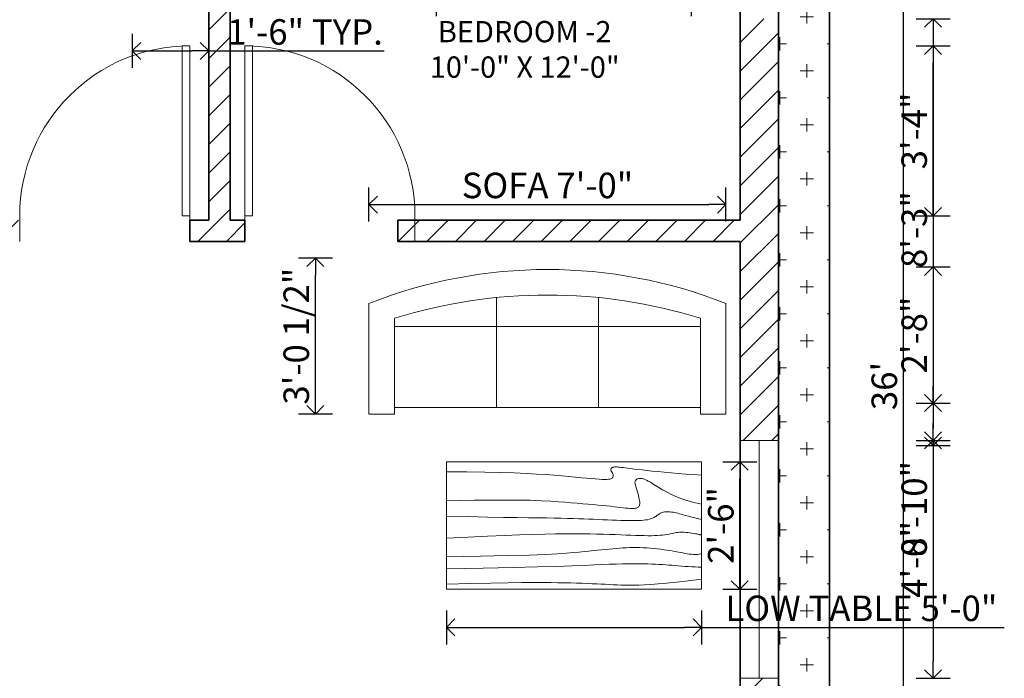
# Model space of a CAD drawing. Units: inches. Extents: x 686 to 1065, y 83 to 664.
# Tile 4 of 5: x 833 to 1065, y 308 to 463. Entities that reach past the tile are written whole.
import ezdxf

# ---------------------------------------------------------------- set-up
doc = ezdxf.new("R2010")
doc.units = ezdxf.units.IN
for name, color, linetype, lineweight in [('A-ANNO-DIMS', 2, 'Continuous', 18), ('A-AREA-IDEN', 7, 'Continuous', 20), ('A-DOOR', 4, 'Continuous', 20), ('A-FURN', 8, 'Continuous', 18), ('A-GLAZ', 172, 'Continuous', 18), ('A-WALL', 7, 'Continuous', 35), ('A-WALL-PATT', 253, 'Continuous', 13), ('C-PROP', 7, 'Continuous', 35), ('L-SITE-PATT', 94, 'Continuous', 13)]:
    doc.layers.add(name, color=color, linetype=linetype, lineweight=lineweight)
doc.styles.get("Standard").update_dxf_attribs({"font": 'arial.ttf'})
doc.dimstyles.new('ISO-25', dxfattribs={"dimtxt": 6, "dimasz": 4, "dimexe": 4, "dimexo": 4, "dimtad": 1, "dimdec": 1, "dimlunit": 3, "dimtxsty": 'Standard', "dimblk": 'OPEN90', "dimcen": 2.5, "dimadec": 0, "dimazin": 0, "dimtfac": 1, "dimtdec": 1, "dimtmove": 0, "dimatfit": 3, "dimfxl": 4, "dimfxlon": 1, "dimarcsym": 0})

# ---------------------------------------------------------------- blocks, each defined once
blk = doc.blocks.new('Sofa - Roundback 7 ft.')
for p, q in [((-12.00002, -32.4421), (-12.00003, -6.5971)), ((11.99997, -32.4421), (11.99998, -6.5971)), ((-36.000027, -34), (-36.000027, -11.4696)), ((35.99998, -34), (35.99998, -11.4696)), ((-35.999844, -13.3819), (35.9998, -13.3819)), ((-36.000027, -32.4421), (35.99998, -32.4421))]:
    blk.add_line(p, q)
for points in [[(-36.000027, -34), (-42.000027, -34), (-42.000027, -8)], [(41.99998, -8), (41.99998, -34), (35.99998, -34)]]:
    blk.add_lwpolyline(points)
for centre, radius, start, end in [((0, -114.25), 114.25, 68.43141, 111.5686), ((-0.00001, -127.1968), 121.1968, 72.72033, 107.2797)]:
    blk.add_arc(centre, radius, start, end)
blk = doc.blocks.new('Table - Rectangular Woodgrain 60 x 30 in.')
for p, q in [((0, 0), (0, -30)), ((60, 0), (0, 0)), ((60, -30), (60, 0)), ((0, -30), (60, -30))]:
    blk.add_line(p, q)
for points in [[(0, -2.4), (4.8155, -2.418), (9.0302, -2.4688), (12.709, -2.5477), (15.9167, -2.65), (18.7181, -2.7711), (21.1781, -2.9063), (23.3616, -3.0508), (25.3333, -3.2), (27.1477, -3.3495), (28.8172, -3.4958), (30.3437, -3.636), (31.7291, -3.7667), (32.9756, -3.8849), (34.0849, -3.9875), (35.059, -4.0714), (35.9, -4.1334), (36.6114, -4.1711), (37.2041, -4.1854), (37.6906, -4.1779), (38.0833, -4.15), (38.3948, -4.1034), (38.6375, -4.0396), (38.8239, -3.9602), (38.9666, -3.8667), (39.0764, -3.7608), (39.1573, -3.6448), (39.2116, -3.521), (39.2416, -3.3917), (39.2498, -3.2593), (39.2385, -3.1261), (39.21, -2.9944), (39.1666, -2.8667), (39.111, -2.7447), (39.0468, -2.6281), (38.978, -2.5163), (38.9083, -2.4083), (38.8418, -2.3035), (38.7823, -2.201), (38.7337, -2.1001), (38.7, -2), (38.6844, -1.9003), (38.6875, -1.8021), (38.7094, -1.707), (38.75, -1.6167), (38.8094, -1.5326), (38.8875, -1.4563), (38.9844, -1.3893), (39.1, -1.3333), (39.2351, -1.2896), (39.3937, -1.2583), (39.5804, -1.2396), (39.8, -1.2333), (40.057, -1.2396), (40.3562, -1.2583), (40.7023, -1.2896), (41.1, -1.3333), (41.5547, -1.3895), (42.0755, -1.4573), (42.6721, -1.5361), (43.3542, -1.625), (44.1316, -1.7233), (45.014, -1.8302), (46.0114, -1.9449), (47.1333, -2.0667), (48.3862, -2.1947), (49.7625, -2.3281), (51.2513, -2.4663), (52.8416, -2.6083), (54.5226, -2.7535), (56.2833, -2.9011), (58.1127, -3.0501), (60, -3.2)], [(0, -9.2), (6.5759, -9.0858), (11.9385, -9.0365), (16.2527, -9.0418), (19.6833, -9.0917), (22.3952, -9.1759), (24.5531, -9.2844), (26.322, -9.4069), (27.8666, -9.5333), (29.3241, -9.6553), (30.7203, -9.7719), (32.0532, -9.8837), (33.3208, -9.9917), (34.5213, -10.0965), (35.6526, -10.199), (36.7128, -10.2999), (37.7, -10.4), (38.6129, -10.4996), (39.4531, -10.5969), (40.223, -10.6895), (40.925, -10.775), (41.5613, -10.8512), (42.1344, -10.9156), (42.6465, -10.966), (43.1, -11), (43.4976, -11.0158), (43.8437, -11.0136), (44.143, -10.9942), (44.4, -10.9583), (44.6195, -10.9069), (44.8062, -10.8406), (44.9648, -10.7603), (45.1, -10.6667), (45.2155, -10.5598), (45.3114, -10.4365), (45.3871, -10.2929), (45.4416, -10.125), (45.4743, -9.929), (45.4844, -9.7011), (45.4709, -9.4371), (45.4333, -9.1333), (45.3716, -8.7883), (45.2896, -8.4104), (45.1919, -8.0107), (45.0833, -7.6), (44.9685, -7.1893), (44.8521, -6.7896), (44.7388, -6.4117), (44.6333, -6.0667), (44.54, -5.7628), (44.4614, -5.4979), (44.4001, -5.2675), (44.3583, -5.0667), (44.3384, -4.8909), (44.3427, -4.7354), (44.3736, -4.5956), (44.4333, -4.4667), (44.5236, -4.3453), (44.6427, -4.2333), (44.7884, -4.1339), (44.9583, -4.05), (45.1501, -3.9849), (45.3614, -3.9417), (45.59, -3.9234), (45.8333, -3.9333), (46.0915, -3.9749), (46.3734, -4.0531), (46.6906, -4.1736), (47.0542, -4.3417), (47.4756, -4.5629), (47.9661, -4.8427), (48.5372, -5.1866), (49.2, -5.6), (49.9676, -6.0844), (50.8594, -6.625), (51.8965, -7.2031), (53.1, -7.8), (54.491, -8.3969), (56.0906, -8.975), (57.9199, -9.5156), (60, -10)], [(0, -12.8), (5.1847, -12.9322), (9.6213, -13.0323), (13.3963, -13.1059), (16.5958, -13.1583), (19.3063, -13.1952), (21.614, -13.2219), (23.6054, -13.2439), (25.3666, -13.2667), (26.9728, -13.2947), (28.4531, -13.3281), (29.8256, -13.3663), (31.1083, -13.4083), (32.3191, -13.4535), (33.476, -13.501), (34.597, -13.5501), (35.7, -13.6), (36.7984, -13.6497), (37.8875, -13.6979), (38.9578, -13.743), (40, -13.7833), (41.0047, -13.8174), (41.9625, -13.8438), (42.864, -13.8607), (43.7, -13.8667), (44.4631, -13.8604), (45.1552, -13.8417), (45.7801, -13.8104), (46.3416, -13.7667), (46.8439, -13.7104), (47.2906, -13.6417), (47.6858, -13.5604), (48.0333, -13.4667), (48.3375, -13.3608), (48.6042, -13.2448), (48.8396, -13.121), (49.05, -12.9917), (49.2417, -12.8593), (49.4208, -12.7261), (49.5937, -12.5944), (49.7667, -12.4667), (49.9452, -12.3451), (50.1323, -12.2313), (50.3303, -12.1268), (50.5416, -12.0333), (50.7686, -11.9524), (51.0135, -11.8854), (51.2788, -11.8341), (51.5666, -11.8), (51.8785, -11.7843), (52.2116, -11.7865), (52.562, -11.8059), (52.926, -11.8417), (53.2998, -11.8931), (53.6795, -11.9594), (54.0614, -12.0397), (54.4416, -12.1333), (54.8223, -12.2401), (55.2293, -12.3625), (55.6942, -12.5037), (56.2489, -12.6667), (56.9251, -12.8547), (57.7545, -13.0708), (58.7689, -13.3182), (60, -13.6)], [(0, -18), (5.124, -17.7273), (9.6609, -17.5057), (13.6705, -17.3303), (17.2125, -17.1958), (20.3467, -17.0973), (23.1328, -17.0297), (25.6307, -16.9878), (27.9, -16.9667), (29.9928, -16.9617), (31.9302, -16.9703), (33.7254, -16.9907), (35.3917, -17.0208), (36.9423, -17.0588), (38.3906, -17.1026), (39.7499, -17.1503), (41.0333, -17.2), (42.2519, -17.2496), (43.4073, -17.2969), (44.4986, -17.3395), (45.525, -17.375), (46.4858, -17.4012), (47.3802, -17.4156), (48.2074, -17.416), (48.9667, -17.4), (49.6583, -17.3662), (50.2872, -17.3167), (50.8595, -17.2547), (51.3812, -17.1833), (51.8584, -17.1057), (52.2971, -17.025), (52.7034, -16.9443), (53.0833, -16.8667), (53.443, -16.7951), (53.789, -16.7313), (54.128, -16.6768), (54.4666, -16.6334), (54.8115, -16.6024), (55.1693, -16.5854), (55.5465, -16.5841), (55.95, -16.6), (56.3828, -16.6337), (56.8346, -16.6823), (57.2915, -16.7418), (57.7396, -16.8084), (58.165, -16.878), (58.5539, -16.9469), (58.8924, -17.0111), (59.1666, -17.0667), (59.3679, -17.1107), (59.5078, -17.1438), (59.6032, -17.1675), (59.6708, -17.1833), (59.7275, -17.193), (59.7901, -17.1979), (59.8753, -17.1998), (60, -17.2)], [(0, -22.4), (8.0098, -22.2501), (14.4094, -22.1011), (19.4168, -21.9535), (23.25, -21.8083), (26.1269, -21.6663), (28.2656, -21.5281), (29.884, -21.3947), (31.2, -21.2667), (32.3967, -21.1448), (33.5172, -21.0292), (34.5697, -20.9198), (35.5625, -20.8167), (36.5037, -20.7198), (37.4015, -20.6292), (38.2642, -20.5448), (39.1, -20.4667), (39.9164, -20.3951), (40.7187, -20.3313), (41.5117, -20.2768), (42.3, -20.2333), (43.0883, -20.2024), (43.8812, -20.1854), (44.6836, -20.1841), (45.5, -20.2), (46.3328, -20.234), (47.1747, -20.2844), (48.0163, -20.3488), (48.8479, -20.425), (49.66, -20.5106), (50.4429, -20.6031), (51.1872, -20.7004), (51.8833, -20.8), (52.5246, -20.8999), (53.1166, -20.9995), (53.6681, -21.0983), (54.1875, -21.1958), (54.6834, -21.2919), (55.1646, -21.3859), (55.6394, -21.4777), (56.1167, -21.5667), (56.6028, -21.6515), (57.0961, -21.7266), (57.5929, -21.7852), (58.0896, -21.8208), (58.5823, -21.8268), (59.0674, -21.7964), (59.5412, -21.723), (60, -21.6)], [(0, -25.2), (8.6355, -25.0504), (15.7026, -24.9031), (21.4049, -24.7606), (25.9458, -24.625), (29.529, -24.4988), (32.3578, -24.3844), (34.6359, -24.284), (36.5667, -24.2), (38.3213, -24.1341), (39.9417, -24.0854), (41.437, -24.0523), (42.8167, -24.0333), (44.0901, -24.0268), (45.2667, -24.0313), (46.3557, -24.0451), (47.3667, -24.0667), (48.309, -24.0947), (49.1928, -24.1287), (50.0284, -24.168), (50.826, -24.2125), (51.5959, -24.2617), (52.3483, -24.3151), (53.0935, -24.3725), (53.8417, -24.4334), (54.6009, -24.497), (55.3699, -24.561), (56.1454, -24.6226), (56.9239, -24.6792), (57.7021, -24.7279), (58.4764, -24.7662), (59.2435, -24.7911), (60, -24.8)], [(0, -28.8), (5.6867, -28.6681), (10.45, -28.5698), (14.407, -28.5012), (17.675, -28.4584), (20.3711, -28.4374), (22.6125, -28.4344), (24.5164, -28.4455), (26.2, -28.4667), (27.762, -28.4947), (29.2276, -28.5281), (30.6033, -28.5663), (31.8958, -28.6084), (33.1118, -28.6535), (34.2578, -28.7011), (35.3405, -28.7501), (36.3666, -28.8), (37.3443, -28.8497), (38.288, -28.8974), (39.2137, -28.9412), (40.1375, -28.9792), (41.0753, -29.0093), (42.0432, -29.0297), (43.0572, -29.0384), (44.1333, -29.0333), (45.2936, -29.0114), (46.5843, -28.9641), (48.0579, -28.8816), (49.7666, -28.7542), (51.7629, -28.5721), (54.0989, -28.3255), (56.8272, -28.0048), (60, -27.6)]]:
    blk.add_lwpolyline(points)
blk = doc.blocks.new('_Open90')
at = {"color": 0, "linetype": 'ByBlock', "lineweight": -2}
for p, q in [((0, 0), (-1, 0)), ((-0.5, 0.5), (0, 0)), ((0, 0), (-0.5, -0.5))]:
    blk.add_line(p, q, dxfattribs=at)
blk = doc.blocks.new('*D8')
at = {"layer": 'A-ANNO-DIMS', "color": 0, "lineweight": -2, "transparency": 16777216}
for p, q in [((1036.76, 592.73), (1044.76, 592.73)), ((1040.76, 588.73), (1040.76, 164.73)), ((1036.76, 160.73), (1044.76, 160.73))]:
    blk.add_line(p, q, dxfattribs=at)
at = {"layer": 'Defpoints', "color": 0, "transparency": 16777216}
for p in [(1023.37, 592.73), (1023.37, 160.73), (1040.76, 160.73)]:
    blk.add_point(p, dxfattribs=at)
at = {"layer": 'A-ANNO-DIMS', "color": 0, "lineweight": -2, "transparency": 16777216, "xscale": 4, "yscale": 4, "zscale": 4}
for p, rotation in [((1040.76, 592.73), 90), ((1040.76, 160.73), 270)]:
    blk.add_blockref('_Open90', p, dxfattribs=dict(at, rotation=rotation))
at = {"layer": 'A-ANNO-DIMS', "color": 0, "transparency": 16777216, "insert": (1037.07, 376.73), "char_height": 6, "attachment_point": 5, "rotation": 90}
blk.add_mtext("36'", dxfattribs=at)
blk = doc.blocks.new('*U23')
for p, q in [((0, 0), (0, -6)), ((-40, 0), (-40, -6))]:
    blk.add_line(p, q)
blk.add_lwpolyline([(0, 0), (0, 40), (-1.75, 40), (-1.75, 0)], close=True)
blk.add_arc((0, 0), 40, 90, 180)
blk = doc.blocks.new('*D27')
at = {"layer": 'A-ANNO-DIMS', "color": 0, "lineweight": -2, "transparency": 16777216}
for p, q in [((930.83, 471.73), (930.83, 463.73)), ((990.83, 471.73), (990.83, 463.73)), ((986.83, 467.73), (934.83, 467.73))]:
    blk.add_line(p, q, dxfattribs=at)
at = {"layer": 'Defpoints', "color": 0, "transparency": 16777216}
for p in [(930.83, 479.73), (990.83, 479.73), (930.83, 467.73)]:
    blk.add_point(p, dxfattribs=at)
at = {"layer": 'A-ANNO-DIMS', "color": 0, "lineweight": -2, "transparency": 16777216, "xscale": 4, "yscale": 4, "zscale": 4, "rotation": 180}
blk.add_blockref('_Open90', (930.83, 467.73), dxfattribs=at)
at = {"layer": 'A-ANNO-DIMS', "color": 0, "lineweight": -2, "transparency": 16777216, "xscale": 4, "yscale": 4, "zscale": 4}
blk.add_blockref('_Open90', (990.83, 467.73), dxfattribs=at)
at = {"layer": 'A-ANNO-DIMS', "color": 0, "transparency": 16777216, "insert": (960.83, 471.42), "char_height": 6, "attachment_point": 5}
blk.add_mtext('5\'-0" TYP.', dxfattribs=at)
blk = doc.blocks.new('*D29')
at = {"layer": 'A-ANNO-DIMS', "color": 0, "lineweight": -2, "transparency": 16777216}
for p, q in [((859.37, 459.54), (859.37, 451.54)), ((877.37, 459.54), (877.37, 451.54)), ((863.37, 455.54), (873.37, 455.54)), ((877.37, 455.54), (918.63, 455.54))]:
    blk.add_line(p, q, dxfattribs=at)
at = {"layer": 'Defpoints', "color": 0, "transparency": 16777216}
for p in [(859.37, 468.63), (877.37, 468.63), (877.37, 455.54)]:
    blk.add_point(p, dxfattribs=at)
at = {"layer": 'A-ANNO-DIMS', "color": 0, "lineweight": -2, "transparency": 16777216, "xscale": 4, "yscale": 4, "zscale": 4, "rotation": 180}
blk.add_blockref('_Open90', (859.37, 455.54), dxfattribs=at)
at = {"layer": 'A-ANNO-DIMS', "color": 0, "lineweight": -2, "transparency": 16777216, "xscale": 4, "yscale": 4, "zscale": 4}
blk.add_blockref('_Open90', (877.37, 455.54), dxfattribs=at)
at = {"layer": 'A-ANNO-DIMS', "color": 0, "transparency": 16777216, "insert": (900, 459.23), "char_height": 6, "attachment_point": 5}
blk.add_mtext('1\'-6" TYP.', dxfattribs=at)
blk = doc.blocks.new('*D36')
at = {"layer": 'A-ANNO-DIMS', "color": 0, "lineweight": -2, "transparency": 16777216}
for p, q in [((915.04, 415.4), (915.04, 423.4)), ((999.04, 415.4), (999.04, 423.4)), ((919.04, 419.4), (995.04, 419.4))]:
    blk.add_line(p, q, dxfattribs=at)
at = {"layer": 'Defpoints', "color": 0, "transparency": 16777216}
for p in [(999.04, 419.4), (915.04, 406.8), (999.04, 406.8)]:
    blk.add_point(p, dxfattribs=at)
at = {"layer": 'A-ANNO-DIMS', "color": 0, "lineweight": -2, "transparency": 16777216, "xscale": 4, "yscale": 4, "zscale": 4, "rotation": 180}
blk.add_blockref('_Open90', (915.04, 419.4), dxfattribs=at)
at = {"layer": 'A-ANNO-DIMS', "color": 0, "lineweight": -2, "transparency": 16777216, "xscale": 4, "yscale": 4, "zscale": 4}
blk.add_blockref('_Open90', (999.04, 419.4), dxfattribs=at)
at = {"layer": 'A-ANNO-DIMS', "color": 0, "transparency": 16777216, "insert": (957.04, 423.13), "char_height": 6, "attachment_point": 5}
blk.add_mtext('SOFA 7\'-0"', dxfattribs=at)
blk = doc.blocks.new('*D37')
at = {"layer": 'A-ANNO-DIMS', "color": 0, "lineweight": -2, "transparency": 16777216}
for p, q in [((906.44, 406.8), (898.44, 406.8)), ((902.44, 374.13), (902.44, 402.8)), ((906.44, 370.13), (898.44, 370.13))]:
    blk.add_line(p, q, dxfattribs=at)
at = {"layer": 'Defpoints', "color": 0, "transparency": 16777216}
for p in [(902.44, 406.8), (915.04, 406.8), (915.04, 370.13)]:
    blk.add_point(p, dxfattribs=at)
at = {"layer": 'A-ANNO-DIMS', "color": 0, "lineweight": -2, "transparency": 16777216, "xscale": 4, "yscale": 4, "zscale": 4}
for p, rotation in [((902.44, 406.8), 90), ((902.44, 370.13), 270)]:
    blk.add_blockref('_Open90', p, dxfattribs=dict(at, rotation=rotation))
at = {"layer": 'A-ANNO-DIMS', "color": 0, "transparency": 16777216, "insert": (898.71, 388.46), "char_height": 6, "attachment_point": 5, "rotation": 90}
blk.add_mtext('3\'-0 1/2"', dxfattribs=at)
blk = doc.blocks.new('*D38')
at = {"layer": 'A-ANNO-DIMS', "color": 0, "lineweight": -2, "transparency": 16777216}
for p, q in [((933.28, 323.93), (933.28, 315.93)), ((993.28, 323.93), (993.28, 315.93)), ((937.28, 319.93), (989.28, 319.93)), ((993.28, 319.93), (1064.52, 319.93))]:
    blk.add_line(p, q, dxfattribs=at)
at = {"layer": 'Defpoints', "color": 0, "transparency": 16777216}
for p in [(933.28, 328.93), (993.28, 328.93), (993.28, 319.93)]:
    blk.add_point(p, dxfattribs=at)
at = {"layer": 'A-ANNO-DIMS', "color": 0, "lineweight": -2, "transparency": 16777216, "xscale": 4, "yscale": 4, "zscale": 4, "rotation": 180}
blk.add_blockref('_Open90', (933.28, 319.93), dxfattribs=at)
at = {"layer": 'A-ANNO-DIMS', "color": 0, "lineweight": -2, "transparency": 16777216, "xscale": 4, "yscale": 4, "zscale": 4}
blk.add_blockref('_Open90', (993.28, 319.93), dxfattribs=at)
at = {"layer": 'A-ANNO-DIMS', "color": 0, "transparency": 16777216, "insert": (1030.9, 323.66), "char_height": 6, "attachment_point": 5}
blk.add_mtext('LOW TABLE 5\'-0"', dxfattribs=at)
blk = doc.blocks.new('*D39')
at = {"layer": 'A-ANNO-DIMS', "color": 0, "lineweight": -2, "transparency": 16777216}
for p, q in [((998.28, 358.93), (1006.28, 358.93)), ((1002.28, 332.93), (1002.28, 354.93)), ((998.28, 328.93), (1006.28, 328.93))]:
    blk.add_line(p, q, dxfattribs=at)
at = {"layer": 'Defpoints', "color": 0, "transparency": 16777216}
for p in [(993.28, 358.93), (1002.28, 358.93), (993.28, 328.93)]:
    blk.add_point(p, dxfattribs=at)
at = {"layer": 'A-ANNO-DIMS', "color": 0, "lineweight": -2, "transparency": 16777216, "xscale": 4, "yscale": 4, "zscale": 4}
for p, rotation in [((1002.28, 358.93), 90), ((1002.28, 328.93), 270)]:
    blk.add_blockref('_Open90', p, dxfattribs=dict(at, rotation=rotation))
at = {"layer": 'A-ANNO-DIMS', "color": 0, "transparency": 16777216, "insert": (998.59, 343.93), "char_height": 6, "attachment_point": 5, "rotation": 90}
blk.add_mtext('2\'-6"', dxfattribs=at)
blk = doc.blocks.new('*D48')
at = {"layer": 'A-ANNO-DIMS', "color": 0, "lineweight": -2, "transparency": 16777216}
for p, q in [((1043.78, 463.11), (1051.78, 463.11)), ((1047.78, 459.11), (1047.78, 367.95)), ((1043.78, 363.95), (1051.78, 363.95))]:
    blk.add_line(p, q, dxfattribs=at)
at = {"layer": 'Defpoints', "color": 0, "transparency": 16777216}
for p in [(1011.37, 463.11), (1011.37, 363.95), (1047.78, 363.95)]:
    blk.add_point(p, dxfattribs=at)
at = {"layer": 'A-ANNO-DIMS', "color": 0, "lineweight": -2, "transparency": 16777216, "xscale": 4, "yscale": 4, "zscale": 4}
for p, rotation in [((1047.78, 463.11), 90), ((1047.78, 363.95), 270)]:
    blk.add_blockref('_Open90', p, dxfattribs=dict(at, rotation=rotation))
at = {"layer": 'A-ANNO-DIMS', "color": 0, "transparency": 16777216, "insert": (1044.09, 413.53), "char_height": 6, "attachment_point": 5, "rotation": 90}
blk.add_mtext('8\'-3"', dxfattribs=at)
blk = doc.blocks.new('*D49')
at = {"layer": 'A-ANNO-DIMS', "color": 0, "lineweight": -2, "transparency": 16777216}
for p, q in [((1043.78, 363.95), (1051.78, 363.95)), ((1047.78, 359.95), (1047.78, 311.98)), ((1043.78, 307.98), (1051.78, 307.98))]:
    blk.add_line(p, q, dxfattribs=at)
at = {"layer": 'Defpoints', "color": 0, "transparency": 16777216}
for p in [(1011.37, 363.95), (1011.37, 307.98), (1047.78, 307.98)]:
    blk.add_point(p, dxfattribs=at)
at = {"layer": 'A-ANNO-DIMS', "color": 0, "lineweight": -2, "transparency": 16777216, "xscale": 4, "yscale": 4, "zscale": 4}
for p, rotation in [((1047.78, 363.95), 90), ((1047.78, 307.98), 270)]:
    blk.add_blockref('_Open90', p, dxfattribs=dict(at, rotation=rotation))
at = {"layer": 'A-ANNO-DIMS', "color": 0, "transparency": 16777216, "insert": (1044.09, 335.96), "char_height": 6, "attachment_point": 5, "rotation": 90}
blk.add_mtext('4\'-8"', dxfattribs=at)
blk = doc.blocks.new('*D54')
at = {"layer": 'A-ANNO-DIMS', "color": 0, "lineweight": -2, "transparency": 16777216}
for p, q in [((832.87, 613.14), (832.87, 621.14)), ((872.87, 613.14), (872.87, 621.14)), ((836.87, 617.14), (868.87, 617.14))]:
    blk.add_line(p, q, dxfattribs=at)
at = {"layer": 'Defpoints', "color": 0, "transparency": 16777216}
for p in [(872.87, 617.14), (832.87, 415.73), (872.87, 415.73)]:
    blk.add_point(p, dxfattribs=at)
at = {"layer": 'A-ANNO-DIMS', "color": 0, "lineweight": -2, "transparency": 16777216, "xscale": 4, "yscale": 4, "zscale": 4, "rotation": 180}
blk.add_blockref('_Open90', (832.87, 617.14), dxfattribs=at)
at = {"layer": 'A-ANNO-DIMS', "color": 0, "lineweight": -2, "transparency": 16777216, "xscale": 4, "yscale": 4, "zscale": 4}
blk.add_blockref('_Open90', (872.87, 617.14), dxfattribs=at)
at = {"layer": 'A-ANNO-DIMS', "color": 0, "transparency": 16777216, "insert": (852.87, 620.83), "char_height": 6, "attachment_point": 5}
blk.add_mtext('3\'-4"', dxfattribs=at)
blk = doc.blocks.new('*D55')
at = {"layer": 'A-ANNO-DIMS', "color": 0, "lineweight": -2, "transparency": 16777216}
for p, q in [((885.87, 613.14), (885.87, 621.14)), ((921.87, 613.14), (921.87, 621.14)), ((889.87, 617.14), (917.87, 617.14))]:
    blk.add_line(p, q, dxfattribs=at)
at = {"layer": 'Defpoints', "color": 0, "transparency": 16777216}
for p in [(921.87, 617.14), (885.87, 415.73), (921.87, 415.73)]:
    blk.add_point(p, dxfattribs=at)
at = {"layer": 'A-ANNO-DIMS', "color": 0, "lineweight": -2, "transparency": 16777216, "xscale": 4, "yscale": 4, "zscale": 4, "rotation": 180}
blk.add_blockref('_Open90', (885.87, 617.14), dxfattribs=at)
at = {"layer": 'A-ANNO-DIMS', "color": 0, "lineweight": -2, "transparency": 16777216, "xscale": 4, "yscale": 4, "zscale": 4}
blk.add_blockref('_Open90', (921.87, 617.14), dxfattribs=at)
at = {"layer": 'A-ANNO-DIMS', "color": 0, "transparency": 16777216, "insert": (903.87, 620.83), "char_height": 6, "attachment_point": 5}
blk.add_mtext('3\'-0"', dxfattribs=at)
blk = doc.blocks.new('*D56')
at = {"layer": 'A-ANNO-DIMS', "color": 0, "lineweight": -2, "transparency": 16777216}
for p, q in [((900.37, 613.14), (900.37, 621.14)), ((930.37, 613.14), (930.37, 621.14)), ((904.37, 617.14), (926.37, 617.14))]:
    blk.add_line(p, q, dxfattribs=at)
at = {"layer": 'Defpoints', "color": 0, "transparency": 16777216}
for p in [(930.37, 617.14), (900.37, 246.73), (930.37, 246.73)]:
    blk.add_point(p, dxfattribs=at)
at = {"layer": 'A-ANNO-DIMS', "color": 0, "lineweight": -2, "transparency": 16777216, "xscale": 4, "yscale": 4, "zscale": 4, "rotation": 180}
blk.add_blockref('_Open90', (900.37, 617.14), dxfattribs=at)
at = {"layer": 'A-ANNO-DIMS', "color": 0, "lineweight": -2, "transparency": 16777216, "xscale": 4, "yscale": 4, "zscale": 4}
blk.add_blockref('_Open90', (930.37, 617.14), dxfattribs=at)
at = {"layer": 'A-ANNO-DIMS', "color": 0, "transparency": 16777216, "insert": (915.37, 620.83), "char_height": 6, "attachment_point": 5}
blk.add_mtext('2\'-6"', dxfattribs=at)
blk = doc.blocks.new('*D57')
at = {"layer": 'A-ANNO-DIMS', "color": 0, "lineweight": -2, "transparency": 16777216}
for p, q in [((1043.78, 404.73), (1051.78, 404.73)), ((1047.78, 400.73), (1047.78, 376.73)), ((1043.78, 372.73), (1051.78, 372.73))]:
    blk.add_line(p, q, dxfattribs=at)
at = {"layer": 'Defpoints', "color": 0, "transparency": 16777216}
for p in [(828.37, 404.73), (828.37, 372.73), (1047.78, 372.73)]:
    blk.add_point(p, dxfattribs=at)
at = {"layer": 'A-ANNO-DIMS', "color": 0, "lineweight": -2, "transparency": 16777216, "xscale": 4, "yscale": 4, "zscale": 4}
for p, rotation in [((1047.78, 404.73), 90), ((1047.78, 372.73), 270)]:
    blk.add_blockref('_Open90', p, dxfattribs=dict(at, rotation=rotation))
at = {"layer": 'A-ANNO-DIMS', "color": 0, "transparency": 16777216, "insert": (1044.09, 388.73), "char_height": 6, "attachment_point": 5, "rotation": 90}
blk.add_mtext('2\'-8"', dxfattribs=at)
blk = doc.blocks.new('*D61')
at = {"layer": 'A-ANNO-DIMS', "color": 0, "lineweight": -2, "transparency": 16777216}
for p, q in [((1043.78, 372.73), (1051.78, 372.73)), ((1047.78, 368.73), (1047.78, 366.73)), ((1043.78, 362.73), (1051.78, 362.73)), ((1047.78, 362.73), (1047.78, 336.87))]:
    blk.add_line(p, q, dxfattribs=at)
at = {"layer": 'Defpoints', "color": 0, "transparency": 16777216}
for p in [(823.37, 372.73), (823.37, 362.73), (1047.78, 362.73)]:
    blk.add_point(p, dxfattribs=at)
at = {"layer": 'A-ANNO-DIMS', "color": 0, "lineweight": -2, "transparency": 16777216, "xscale": 4, "yscale": 4, "zscale": 4}
for p, rotation in [((1047.78, 372.73), 90), ((1047.78, 362.73), 270)]:
    blk.add_blockref('_Open90', p, dxfattribs=dict(at, rotation=rotation))
at = {"layer": 'A-ANNO-DIMS', "color": 0, "transparency": 16777216, "insert": (1044.09, 347.8), "char_height": 6, "attachment_point": 5, "rotation": 90}
blk.add_mtext('0\'-10"', dxfattribs=at)
blk = doc.blocks.new('*D63')
at = {"layer": 'A-ANNO-DIMS', "color": 0, "lineweight": -2, "transparency": 16777216}
for p, q in [((823.37, 92.32), (823.37, 84.32)), ((828.37, 92.32), (828.37, 84.32)), ((819.37, 88.32), (815.37, 88.32)), ((823.37, 88.32), (828.37, 88.32)), ((832.37, 88.32), (853.57, 88.32))]:
    blk.add_line(p, q, dxfattribs=at)
at = {"layer": 'Defpoints', "color": 0, "transparency": 16777216}
for p in [(823.37, 362.73), (828.37, 357.73), (828.37, 88.32)]:
    blk.add_point(p, dxfattribs=at)
at = {"layer": 'A-ANNO-DIMS', "color": 0, "lineweight": -2, "transparency": 16777216, "xscale": 4, "yscale": 4, "zscale": 4}
blk.add_blockref('_Open90', (823.37, 88.32), dxfattribs=at)
at = {"layer": 'A-ANNO-DIMS', "color": 0, "lineweight": -2, "transparency": 16777216, "xscale": 4, "yscale": 4, "zscale": 4, "rotation": 180}
blk.add_blockref('_Open90', (828.37, 88.32), dxfattribs=at)
at = {"layer": 'A-ANNO-DIMS', "color": 0, "transparency": 16777216, "insert": (844.97, 92.01), "char_height": 6, "attachment_point": 5}
blk.add_mtext('0\'-5"', dxfattribs=at)
blk = doc.blocks.new('*D64')
at = {"layer": 'A-ANNO-DIMS', "color": 0, "lineweight": -2, "transparency": 16777216}
for p, q in [((872.87, 92.32), (872.87, 84.32)), ((877.37, 92.32), (877.37, 84.32)), ((868.87, 88.32), (864.87, 88.32)), ((872.87, 88.32), (877.37, 88.32)), ((881.37, 88.32), (916.55, 88.32))]:
    blk.add_line(p, q, dxfattribs=at)
at = {"layer": 'Defpoints', "color": 0, "transparency": 16777216}
for p in [(877.37, 415.73), (872.87, 410.73), (877.37, 88.32)]:
    blk.add_point(p, dxfattribs=at)
at = {"layer": 'A-ANNO-DIMS', "color": 0, "lineweight": -2, "transparency": 16777216, "xscale": 4, "yscale": 4, "zscale": 4}
blk.add_blockref('_Open90', (872.87, 88.32), dxfattribs=at)
at = {"layer": 'A-ANNO-DIMS', "color": 0, "lineweight": -2, "transparency": 16777216, "xscale": 4, "yscale": 4, "zscale": 4, "rotation": 180}
blk.add_blockref('_Open90', (877.37, 88.32), dxfattribs=at)
at = {"layer": 'A-ANNO-DIMS', "color": 0, "transparency": 16777216, "insert": (900.96, 92.05), "char_height": 6, "attachment_point": 5}
blk.add_mtext('0\'-4 1/2"', dxfattribs=at)
blk = doc.blocks.new('*D65')
at = {"layer": 'A-ANNO-DIMS', "color": 0, "lineweight": -2, "transparency": 16777216}
for p, q in [((882.37, 92.32), (882.37, 84.32)), ((885.87, 92.32), (885.87, 84.32)), ((878.37, 88.32), (874.37, 88.32)), ((882.37, 88.32), (885.87, 88.32)), ((889.87, 88.32), (925.05, 88.32))]:
    blk.add_line(p, q, dxfattribs=at)
at = {"layer": 'Defpoints', "color": 0, "transparency": 16777216}
for p in [(882.37, 415.73), (885.87, 410.73), (885.87, 88.32)]:
    blk.add_point(p, dxfattribs=at)
at = {"layer": 'A-ANNO-DIMS', "color": 0, "lineweight": -2, "transparency": 16777216, "xscale": 4, "yscale": 4, "zscale": 4}
blk.add_blockref('_Open90', (882.37, 88.32), dxfattribs=at)
at = {"layer": 'A-ANNO-DIMS', "color": 0, "lineweight": -2, "transparency": 16777216, "xscale": 4, "yscale": 4, "zscale": 4, "rotation": 180}
blk.add_blockref('_Open90', (885.87, 88.32), dxfattribs=at)
at = {"layer": 'A-ANNO-DIMS', "color": 0, "transparency": 16777216, "insert": (909.46, 92.05), "char_height": 6, "attachment_point": 5}
blk.add_mtext('0\'-3 1/2"', dxfattribs=at)
blk = doc.blocks.new('*D66')
at = {"layer": 'A-ANNO-DIMS', "color": 0, "lineweight": -2, "transparency": 16777216}
for p, q in [((894.37, 613.14), (894.37, 621.14)), ((900.37, 613.14), (900.37, 621.14)), ((890.37, 617.14), (886.37, 617.14)), ((894.37, 617.14), (900.37, 617.14)), ((904.37, 617.14), (925.57, 617.14))]:
    blk.add_line(p, q, dxfattribs=at)
at = {"layer": 'Defpoints', "color": 0, "transparency": 16777216}
for p in [(900.37, 617.14), (894.37, 241.73), (900.37, 241.73)]:
    blk.add_point(p, dxfattribs=at)
at = {"layer": 'A-ANNO-DIMS', "color": 0, "lineweight": -2, "transparency": 16777216, "xscale": 4, "yscale": 4, "zscale": 4}
blk.add_blockref('_Open90', (894.37, 617.14), dxfattribs=at)
at = {"layer": 'A-ANNO-DIMS', "color": 0, "lineweight": -2, "transparency": 16777216, "xscale": 4, "yscale": 4, "zscale": 4, "rotation": 180}
blk.add_blockref('_Open90', (900.37, 617.14), dxfattribs=at)
at = {"layer": 'A-ANNO-DIMS', "color": 0, "transparency": 16777216, "insert": (916.97, 620.83), "char_height": 6, "attachment_point": 5}
blk.add_mtext('0\'-6"', dxfattribs=at)
blk = doc.blocks.new('*D69')
at = {"layer": 'A-ANNO-DIMS', "color": 0, "lineweight": -2, "transparency": 16777216}
for p, q in [((978.37, 613.14), (978.37, 621.14)), ((1002.37, 613.14), (1002.37, 621.14)), ((982.37, 617.14), (998.37, 617.14))]:
    blk.add_line(p, q, dxfattribs=at)
at = {"layer": 'Defpoints', "color": 0, "transparency": 16777216}
for p in [(1002.37, 617.14), (978.37, 241.73), (1002.37, 241.73)]:
    blk.add_point(p, dxfattribs=at)
at = {"layer": 'A-ANNO-DIMS', "color": 0, "lineweight": -2, "transparency": 16777216, "xscale": 4, "yscale": 4, "zscale": 4, "rotation": 180}
blk.add_blockref('_Open90', (978.37, 617.14), dxfattribs=at)
at = {"layer": 'A-ANNO-DIMS', "color": 0, "lineweight": -2, "transparency": 16777216, "xscale": 4, "yscale": 4, "zscale": 4}
blk.add_blockref('_Open90', (1002.37, 617.14), dxfattribs=at)
at = {"layer": 'A-ANNO-DIMS', "color": 0, "transparency": 16777216, "insert": (990.37, 620.83), "char_height": 6, "attachment_point": 5}
blk.add_mtext('2\'-0"', dxfattribs=at)
blk = doc.blocks.new('*D74')
at = {"layer": 'A-ANNO-DIMS', "color": 0, "lineweight": -2, "transparency": 16777216}
for p, q in [((1043.78, 456.73), (1051.78, 456.73)), ((1047.78, 420.73), (1047.78, 452.73)), ((1043.78, 416.73), (1051.78, 416.73))]:
    blk.add_line(p, q, dxfattribs=at)
at = {"layer": 'Defpoints', "color": 0, "transparency": 16777216}
for p in [(887.62, 456.73), (1047.78, 456.73), (887.62, 416.73)]:
    blk.add_point(p, dxfattribs=at)
at = {"layer": 'A-ANNO-DIMS', "color": 0, "lineweight": -2, "transparency": 16777216, "xscale": 4, "yscale": 4, "zscale": 4}
for p, rotation in [((1047.78, 456.73), 90), ((1047.78, 416.73), 270)]:
    blk.add_blockref('_Open90', p, dxfattribs=dict(at, rotation=rotation))
at = {"layer": 'A-ANNO-DIMS', "color": 0, "transparency": 16777216, "insert": (1044.09, 436.73), "char_height": 6, "attachment_point": 5, "rotation": 90}
blk.add_mtext('3\'-4"', dxfattribs=at)
blk = doc.blocks.new('*D75')
at = {"layer": 'A-ANNO-DIMS', "color": 0, "lineweight": -2, "transparency": 16777216}
for p, q in [((841.37, 613.14), (841.37, 621.14)), ((847.37, 613.14), (847.37, 621.14)), ((837.37, 617.14), (833.37, 617.14)), ((841.37, 617.14), (847.37, 617.14)), ((851.37, 617.14), (872.57, 617.14))]:
    blk.add_line(p, q, dxfattribs=at)
at = {"layer": 'Defpoints', "color": 0, "transparency": 16777216}
for p in [(847.37, 617.14), (841.37, 169.73), (847.37, 169.73)]:
    blk.add_point(p, dxfattribs=at)
at = {"layer": 'A-ANNO-DIMS', "color": 0, "lineweight": -2, "transparency": 16777216, "xscale": 4, "yscale": 4, "zscale": 4}
blk.add_blockref('_Open90', (841.37, 617.14), dxfattribs=at)
at = {"layer": 'A-ANNO-DIMS', "color": 0, "lineweight": -2, "transparency": 16777216, "xscale": 4, "yscale": 4, "zscale": 4, "rotation": 180}
blk.add_blockref('_Open90', (847.37, 617.14), dxfattribs=at)
at = {"layer": 'A-ANNO-DIMS', "color": 0, "transparency": 16777216, "insert": (863.97, 620.83), "char_height": 6, "attachment_point": 5}
blk.add_mtext('0\'-6"', dxfattribs=at)

msp = doc.modelspace()

# ---------------------------------------------------------------- hatches: boundary and pattern name
at = {"layer": 'A-WALL-PATT'}
h = msp.add_hatch(dxfattribs=at)
h.set_pattern_fill('ANSI31', color=256, scale=1.5)
h.set_pattern_definition([(45, (464.028, 0), (-3.367596, 3.367596), [])])
h.paths.add_polyline_path([(1011.37, 568.73), (742.37, 568.73), (742.37, 499.41), (751.37, 499.41), (751.37, 559.73), (877.37, 559.73), (877.37, 415.73), (872.87, 415.73), (872.87, 410.73), (885.87, 410.73), (885.87, 415.73), (882.37, 415.73), (882.37, 559.73), (1002.37, 559.73), (1002.37, 514.56), (1011.37, 514.56)])
h.paths.add_polyline_path([(832.87, 415.73), (751.37, 415.73), (751.37, 448.47), (742.37, 448.47), (742.37, 397.23), (751.37, 397.23), (751.37, 410.73), (823.37, 410.73), (823.37, 404.73), (828.37, 404.73), (828.37, 410.73), (832.87, 410.73)])
h.paths.add_polyline_path([(751.37, 357.73), (828.37, 357.73), (828.37, 372.73), (823.37, 372.73), (823.37, 362.73), (751.37, 362.73), (751.37, 376.23), (742.37, 376.23), (742.37, 112.73), (751.37, 112.73)])
h.paths.add_polyline_path([(845.37, 160.73), (847.37, 160.73), (847.37, 169.73), (841.37, 169.73), (841.37, 246.73), (836.37, 246.73), (836.37, 117.73), (807.43, 117.73), (807.43, 112.73), (845.37, 112.73)])
h.paths.add_polyline_path([(920.89, 169.73), (904.39, 169.73), (894.37, 169.73), (894.37, 241.73), (900.37, 241.73), (900.37, 246.73), (889.37, 246.73), (889.37, 169.73), (883.37, 169.73), (883.37, 160.73), (920.89, 160.73)])
h.paths.add_polyline_path([(1011.37, 196.2), (1002.37, 196.2), (1002.37, 169.73), (966.91, 169.73), (966.91, 160.73), (1011.37, 160.73)])
h.paths.add_polyline_path([(1011.37, 307.98), (1002.37, 307.98), (1002.37, 232.2), (1011.37, 232.2)])
h.paths.add_polyline_path([(1011.37, 463.11), (1002.37, 463.11), (1002.37, 415.73), (921.87, 415.73), (921.87, 410.73), (1002.37, 410.73), (1002.37, 363.95), (1011.37, 363.95)])
h.paths.add_polyline_path([(781.1, 117.73), (751.37, 117.73), (751.37, 112.73), (781.1, 112.73)], flags=17)
at = {"layer": 'L-SITE-PATT'}
h = msp.add_hatch(dxfattribs=at)
h.set_pattern_fill('CROSS', color=256)
h.set_pattern_definition([(0, (464.028, 0), (6.35, 6.35), [3.175, -9.525]), (90, (465.6154, -1.5875), (-6.35, 6.35), [3.175, -9.525])])
h.paths.add_polyline_path([(742.37, 568.73), (1011.37, 568.73), (1011.37, 160.73), (1023.37, 160.73), (1023.37, 592.73), (723.37, 592.73), (723.37, 112.73), (742.37, 112.73)])
h.paths.add_polyline_path([(1012.48, 266.46), (1021.74, 266.46), (1021.74, 278.82), (1012.48, 278.82)], flags=24)
h.paths.add_polyline_path([(938.61, 576.17), (938.61, 585.43), (926.24, 585.43), (926.24, 576.17)], flags=24)
h.paths.add_polyline_path([(864.77, 570.5), (889.12, 570.5), (889.12, 582.86), (864.77, 582.86)], flags=24)
h.paths.add_polyline_path([(722.77, 199.16), (742.46, 199.16), (742.46, 211.52), (722.77, 211.52)], flags=9)

# ---------------------------------------------------------------- linework, layer by layer
at = {"layer": 'A-GLAZ'}
for p, q in [((1002.37, 363.95), (1011.37, 363.95)), ((1006.87, 363.95), (1006.87, 307.98)), ((1002.37, 307.98), (1011.37, 307.98))]:
    msp.add_line(p, q, dxfattribs=at)
at = {"layer": 'A-WALL'}
for p, q in [((1011.37, 160.73), (1011.37, 568.73)), ((877.37, 559.73), (877.37, 415.73)), ((882.37, 559.73), (882.37, 415.73)), ((1002.37, 415.73), (1002.37, 559.73)), ((877.37, 415.73), (872.87, 415.73)), ((872.87, 410.73), (872.87, 415.73)), ((885.87, 415.73), (882.37, 415.73)), ((885.87, 415.73), (885.87, 410.73)), ((1002.37, 415.73), (921.87, 415.73)), ((921.87, 415.73), (921.87, 410.73)), ((885.87, 410.73), (872.87, 410.73)), ((1002.37, 410.73), (921.87, 410.73)), ((1002.37, 169.73), (1002.37, 410.73))]:
    msp.add_line(p, q, dxfattribs=at)
at = {"layer": 'C-PROP'}
msp.add_line((1023.37, 112.73), (1023.37, 592.73), dxfattribs=at)

# ---------------------------------------------------------------- block references
at = {"layer": 'A-DOOR'}
msp.add_blockref('*U23', (872.87, 416.73), dxfattribs=at)
at = {"layer": 'A-DOOR', "xscale": -1}
msp.add_blockref('*U23', (885.87, 416.73), dxfattribs=at)
at = {"layer": 'A-FURN'}
for name, p in [('Sofa - Roundback 7 ft.', (957.04, 404.13)), ('Table - Rectangular Woodgrain 60 x 30 in.', (933.28, 358.93))]:
    msp.add_blockref(name, p, dxfattribs=at)

# ---------------------------------------------------------------- texts
at = {"layer": 'A-AREA-IDEN', "insert": (920.02, 462.58), "char_height": 5, "attachment_point": 1}
msp.add_mtext_dynamic_manual_height_columns('\\pxqc;BEDROOM -2\\P10\'-0" X 12\'-0"', width=63.3243, gutter_width=12.5, heights=[0], dxfattribs=at)

# ---------------------------------------------------------------- dimensions: what is measured, and where the dimension line sits
at = {"layer": 'A-ANNO-DIMS'}
for base, p1, p2, picture, middle in [((872.87, 617.14), (832.87, 415.73), (872.87, 415.73), '*D54', (852.87, 620.83)), ((847.37, 617.14), (841.37, 169.73), (847.37, 169.73), '*D75', (863.97, 620.83)), ((921.87, 617.14), (885.87, 415.73), (921.87, 415.73), '*D55', (903.87, 620.83)), ((900.37, 617.14), (894.37, 241.73), (900.37, 241.73), '*D66', (916.97, 620.83)), ((930.37, 617.14), (900.37, 246.73), (930.37, 246.73), '*D56', (915.37, 620.83)), ((1002.37, 617.14), (978.37, 241.73), (1002.37, 241.73), '*D69', (990.37, 620.83)), ((877.37, 88.32), (872.87, 410.73), (877.37, 415.73), '*D64', (900.96, 92.05)), ((885.87, 88.32), (882.37, 415.73), (885.87, 410.73), '*D65', (909.46, 92.05)), ((828.37, 88.32), (823.37, 362.73), (828.37, 357.73), '*D63', (844.97, 92.01))]:
    dim = msp.add_linear_dim(base=base, p1=p1, p2=p2, dimstyle='ISO-25', override={"dimdec": 1, "dimlfac": 1, "dimrnd": 0, "dimzin": 1, "dimdsep": 46, "dimlunit": 4, "dimfrac": 2}, dxfattribs=at)
    dim.commit()
    dim.dimension.update_dxf_attribs({"geometry": picture, "text_midpoint": middle})
for base, p1, p2, override, picture, middle in [((1040.76, 160.73), (1023.37, 592.73), (1023.37, 160.73), {"dimclrd": 0, "dimclre": 0, "dimclrt": 0}, '*D8', (1037.07, 376.73)), ((1047.78, 363.95), (1011.37, 463.11), (1011.37, 363.95), {"dimdec": 1, "dimlfac": 1, "dimrnd": 0, "dimzin": 1, "dimdsep": 46, "dimlunit": 4, "dimfrac": 2}, '*D48', (1044.09, 413.53)), ((1047.78, 456.73), (887.62, 416.73), (887.62, 456.73), {"dimdec": 1, "dimlfac": 1, "dimrnd": 0, "dimzin": 1, "dimdsep": 46, "dimlunit": 4, "dimfrac": 2}, '*D74', (1044.09, 436.73)), ((902.44, 406.8), (915.04, 370.13), (915.04, 406.8), {"dimdec": 1, "dimlfac": 1, "dimrnd": 0, "dimzin": 1, "dimdsep": 46, "dimlunit": 4, "dimfrac": 2}, '*D37', (898.71, 388.46)), ((1047.78, 372.73), (828.37, 404.73), (828.37, 372.73), {"dimdec": 1, "dimlfac": 1, "dimrnd": 0, "dimzin": 1, "dimdsep": 46, "dimlunit": 4, "dimfrac": 2}, '*D57', (1044.09, 388.73)), ((1047.78, 362.73), (823.37, 372.73), (823.37, 362.73), {"dimdec": 1, "dimlfac": 1, "dimrnd": 0, "dimzin": 1, "dimdsep": 46, "dimlunit": 4, "dimfrac": 2}, '*D61', (1044.09, 347.8)), ((1047.78, 307.98), (1011.37, 363.95), (1011.37, 307.98), {"dimdec": 1, "dimlfac": 1, "dimrnd": 0, "dimzin": 1, "dimdsep": 46, "dimlunit": 4, "dimfrac": 2}, '*D49', (1044.09, 335.96)), ((1002.28, 358.93), (993.28, 328.93), (993.28, 358.93), {"dimdec": 1, "dimlfac": 1, "dimrnd": 0, "dimzin": 1, "dimdsep": 46, "dimlunit": 4, "dimfrac": 2}, '*D39', (998.59, 343.93))]:
    dim = msp.add_linear_dim(base=base, p1=p1, p2=p2, angle=90, dimstyle='ISO-25', override=override, dxfattribs=at)
    dim.commit()
    dim.dimension.update_dxf_attribs({"geometry": picture, "text_midpoint": middle})
dim = msp.add_linear_dim(base=(930.83, 467.73), p1=(990.83, 479.73), p2=(930.83, 479.73), angle=180, text='<> TYP.', dimstyle='ISO-25', override={"dimdec": 1, "dimlfac": 1, "dimrnd": 0, "dimzin": 1, "dimdsep": 46, "dimlunit": 4, "dimfrac": 2}, dxfattribs=at)
dim.commit()
dim.dimension.update_dxf_attribs({"geometry": '*D27', "text_midpoint": (960.83, 471.42)})
for base, p1, p2, text, picture, middle in [((877.37, 455.54), (859.37, 468.63), (877.37, 468.63), '<> TYP.', '*D29', (900, 459.23)), ((999.04, 419.4), (915.04, 406.8), (999.04, 406.8), 'SOFA <>', '*D36', (957.04, 423.13)), ((993.28, 319.93), (933.28, 328.93), (993.28, 328.93), 'LOW TABLE <>', '*D38', (1030.9, 323.66))]:
    dim = msp.add_linear_dim(base=base, p1=p1, p2=p2, text=text, dimstyle='ISO-25', override={"dimdec": 1, "dimlfac": 1, "dimrnd": 0, "dimzin": 1, "dimdsep": 46, "dimlunit": 4, "dimfrac": 2}, dxfattribs=at)
    dim.commit()
    dim.dimension.update_dxf_attribs({"geometry": picture, "text_midpoint": middle})

doc.saveas('drawing.dxf')
